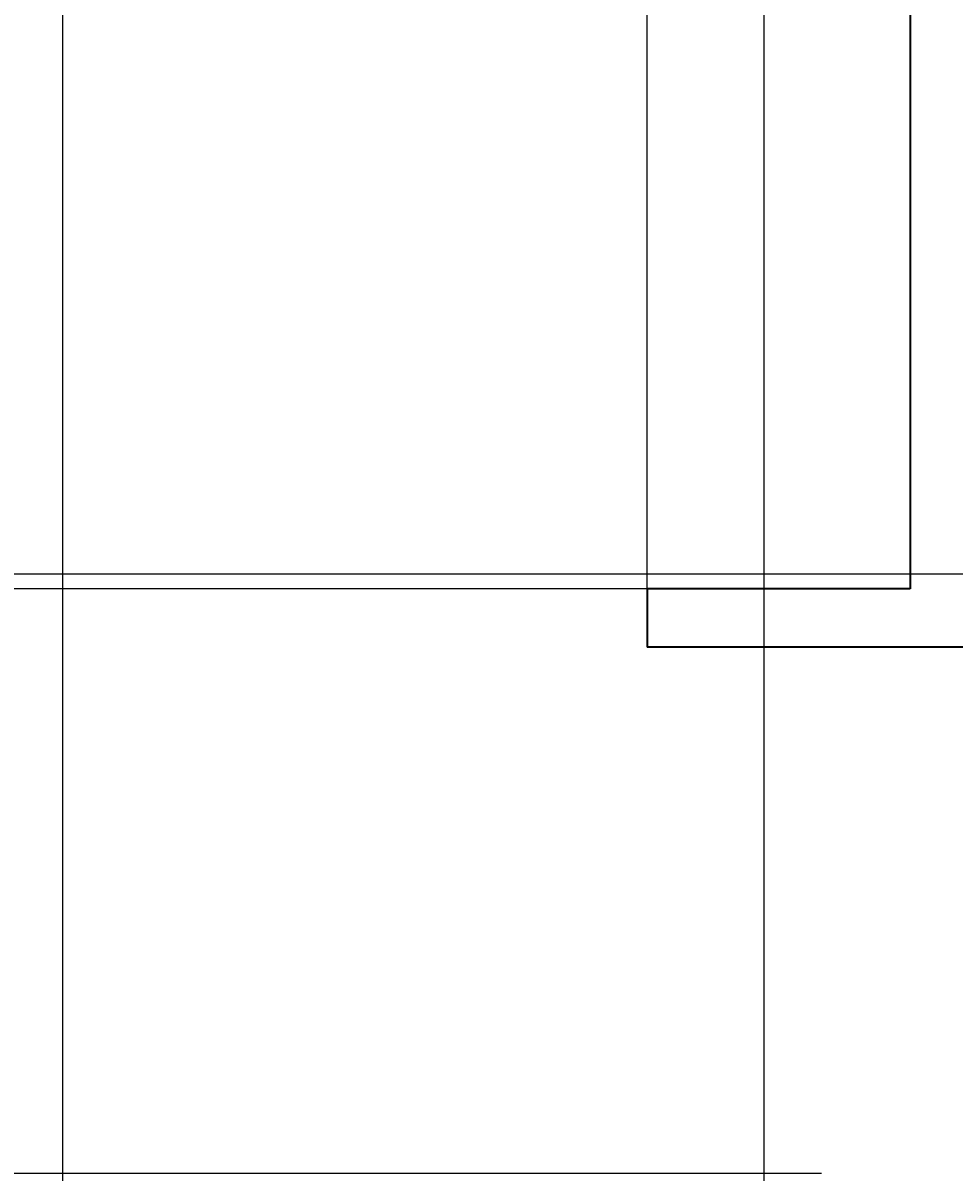
# Model space of a CAD drawing. Units: feet. Extents: x 105 to 1094, y -88 to 588.
# Tile 27 of 59: x 372 to 436, y 354 to 433. Entities that reach past the tile are written whole.
import ezdxf

# ---------------------------------------------------------------- set-up
doc = ezdxf.new("R2010")
doc.units = ezdxf.units.FT
doc.header["$MEASUREMENT"] = 0
doc.layers.add('A-ANNO-DIMS', color=2, linetype='Continuous', lineweight=18)
doc.layers.add('A-WALL', color=7, linetype='Continuous', lineweight=35)
doc.styles.get("Standard").update_dxf_attribs({"font": 'arial.ttf'})
doc.dimstyles.get("Standard").update_dxf_attribs({"dimtxt": 0.18, "dimasz": 0.18, "dimexe": 0.18, "dimexo": 0.0625, "dimgap": 0.09, "dimtad": 0, "dimtih": 1, "dimtoh": 1, "dimdec": 4, "dimzin": 0, "dimdsep": 46, "dimtxsty": 'Standard', "dimcen": 0.09, "dimadec": 0, "dimazin": 0, "dimtfac": 1, "dimtdec": 4, "dimtofl": 0, "dimtmove": 0, "dimatfit": 3, "dimfxl": 1, "dimtolj": 1, "dimtzin": 0, "dimarcsym": 0})

# ---------------------------------------------------------------- blocks, each defined once
blk = doc.blocks.new('*D21')
at = {"layer": 'A-ANNO-DIMS', "color": 0, "lineweight": -2, "transparency": 16777216}
for p, q in [((849.626, 543.081), (105.458, 543.081)), ((105.638, 542.901), (105.638, 250.263)), ((105.638, -42.739), (105.638, 249.899)), ((849.626, -42.919), (105.458, -42.919))]:
    blk.add_line(p, q, dxfattribs=at)
at = {"layer": 'A-ANNO-DIMS', "color": 0, "transparency": 16777216}
for points in [[(105.608, 542.901), (105.668, 542.901), (105.638, 543.081)], [(105.608, -42.739), (105.668, -42.739), (105.638, -42.919)]]:
    blk.add_solid(points, dxfattribs=at)
at = {"layer": 'Defpoints', "color": 0, "transparency": 16777216}
for p in [(105.638, 543.081), (849.688, 543.081), (849.688, -42.919)]:
    blk.add_point(p, dxfattribs=at)
at = {"layer": 'A-ANNO-DIMS', "color": 0, "transparency": 16777216, "insert": (105.638, 250.081), "char_height": 0.18, "attachment_point": 5}
blk.add_mtext('\\A1;586', dxfattribs=at)
blk = doc.blocks.new('*D33')
at = {"layer": 'A-ANNO-DIMS', "color": 0, "lineweight": -2, "transparency": 16777216}
for p, q in [((646.626, 395.081), (105.458, 395.081)), ((105.638, 394.901), (105.638, 345.263)), ((105.638, 295.261), (105.638, 344.899)), ((646.626, 295.081), (105.458, 295.081))]:
    blk.add_line(p, q, dxfattribs=at)
at = {"layer": 'A-ANNO-DIMS', "color": 0, "transparency": 16777216}
for points in [[(105.608, 394.901), (105.668, 394.901), (105.638, 395.081)], [(105.608, 295.261), (105.668, 295.261), (105.638, 295.081)]]:
    blk.add_solid(points, dxfattribs=at)
at = {"layer": 'Defpoints', "color": 0, "transparency": 16777216}
for p in [(646.688, 395.081), (105.638, 295.081), (646.688, 295.081)]:
    blk.add_point(p, dxfattribs=at)
at = {"layer": 'A-ANNO-DIMS', "color": 0, "transparency": 16777216, "insert": (105.638, 345.081), "char_height": 0.18, "attachment_point": 5}
blk.add_mtext('\\A1;100', dxfattribs=at)
blk = doc.blocks.new('*D51')
at = {"layer": 'A-ANNO-DIMS', "color": 0, "lineweight": -2, "transparency": 16777216}
for p, q in [((432.626, 394.081), (105.458, 394.081)), ((105.638, 393.901), (105.638, 374.263)), ((105.638, 354.261), (105.638, 373.899)), ((426.626, 354.081), (105.458, 354.081))]:
    blk.add_line(p, q, dxfattribs=at)
at = {"layer": 'A-ANNO-DIMS', "color": 0, "transparency": 16777216}
for points in [[(105.608, 393.901), (105.668, 393.901), (105.638, 394.081)], [(105.608, 354.261), (105.668, 354.261), (105.638, 354.081)]]:
    blk.add_solid(points, dxfattribs=at)
at = {"layer": 'Defpoints', "color": 0, "transparency": 16777216}
for p in [(432.688, 394.081), (105.638, 354.081), (426.688, 354.081)]:
    blk.add_point(p, dxfattribs=at)
at = {"layer": 'A-ANNO-DIMS', "color": 0, "transparency": 16777216, "insert": (105.638, 374.081), "char_height": 0.18, "attachment_point": 5}
blk.add_mtext('\\A1;40', dxfattribs=at)
blk = doc.blocks.new('*D52')
at = {"layer": 'A-ANNO-DIMS', "color": 0, "lineweight": -2, "transparency": 16777216}
for p, q in [((414.688, 394.144), (414.688, 588.311)), ((414.868, 588.131), (423.478, 588.131)), ((432.508, 588.131), (423.899, 588.131)), ((432.688, 394.144), (432.688, 588.311))]:
    blk.add_line(p, q, dxfattribs=at)
at = {"layer": 'A-ANNO-DIMS', "color": 0, "transparency": 16777216}
for points in [[(414.868, 588.161), (414.868, 588.101), (414.688, 588.131)], [(432.508, 588.161), (432.508, 588.101), (432.688, 588.131)]]:
    blk.add_solid(points, dxfattribs=at)
at = {"layer": 'Defpoints', "color": 0, "transparency": 16777216}
for p in [(414.688, 588.131), (414.688, 394.081), (432.688, 394.081)]:
    blk.add_point(p, dxfattribs=at)
at = {"layer": 'A-ANNO-DIMS', "color": 0, "transparency": 16777216, "insert": (423.688, 588.131), "char_height": 0.18, "attachment_point": 5}
blk.add_mtext('\\A1;18', dxfattribs=at)
blk = doc.blocks.new('*D53')
at = {"layer": 'A-ANNO-DIMS', "color": 0, "lineweight": -2, "transparency": 16777216}
for p, q in [((365.688, 394.144), (365.688, 588.311)), ((365.868, 588.131), (389.966, 588.131)), ((414.508, 588.131), (390.411, 588.131)), ((414.688, 394.144), (414.688, 588.311))]:
    blk.add_line(p, q, dxfattribs=at)
at = {"layer": 'A-ANNO-DIMS', "color": 0, "transparency": 16777216}
for points in [[(365.868, 588.161), (365.868, 588.101), (365.688, 588.131)], [(414.508, 588.161), (414.508, 588.101), (414.688, 588.131)]]:
    blk.add_solid(points, dxfattribs=at)
at = {"layer": 'Defpoints', "color": 0, "transparency": 16777216}
for p in [(365.688, 588.131), (365.688, 394.081), (414.688, 394.081)]:
    blk.add_point(p, dxfattribs=at)
at = {"layer": 'A-ANNO-DIMS', "color": 0, "transparency": 16777216, "insert": (390.188, 588.131), "char_height": 0.18, "attachment_point": 5}
blk.add_mtext('\\A1;49', dxfattribs=at)
blk = doc.blocks.new('*D56')
at = {"layer": 'A-ANNO-DIMS', "color": 0, "lineweight": -2, "transparency": 16777216}
for p, q in [((374.688, 252.144), (374.688, 588.311)), ((374.868, 588.131), (398.466, 588.131)), ((422.508, 588.131), (398.911, 588.131)), ((422.688, 252.144), (422.688, 588.311))]:
    blk.add_line(p, q, dxfattribs=at)
at = {"layer": 'A-ANNO-DIMS', "color": 0, "transparency": 16777216}
for points in [[(374.868, 588.161), (374.868, 588.101), (374.688, 588.131)], [(422.508, 588.161), (422.508, 588.101), (422.688, 588.131)]]:
    blk.add_solid(points, dxfattribs=at)
at = {"layer": 'Defpoints', "color": 0, "transparency": 16777216}
for p in [(422.688, 588.131), (374.688, 252.081), (422.688, 252.081)]:
    blk.add_point(p, dxfattribs=at)
at = {"layer": 'A-ANNO-DIMS', "color": 0, "transparency": 16777216, "insert": (398.688, 588.131), "char_height": 0.18, "attachment_point": 5}
blk.add_mtext('\\A1;48', dxfattribs=at)

msp = doc.modelspace()

# ---------------------------------------------------------------- linework, layer by layer
at = {"layer": 'A-WALL'}
for p, q in [((432.6883, 491.0812), (432.6883, 394.0812)), ((432.6883, 394.0812), (414.6883, 394.0812)), ((414.6883, 394.0812), (414.6883, 390.0812)), ((436.6883, 390.0812), (414.6883, 390.0812))]:
    msp.add_line(p, q, dxfattribs=at)

# ---------------------------------------------------------------- dimensions: what is measured, and where the dimension line sits
at = {"layer": 'A-ANNO-DIMS'}
for base, p1, p2, picture, middle in [((365.6883, 588.1312), (414.6883, 394.0812), (365.6883, 394.0812), '*D53', (390.1883, 588.1312)), ((422.6883, 588.1312), (374.6883, 252.0812), (422.6883, 252.0812), '*D56', (398.6883, 588.1312)), ((414.6883, 588.1312), (432.6883, 394.0812), (414.6883, 394.0812), '*D52', (423.6883, 588.1312))]:
    dim = msp.add_linear_dim(base=base, p1=p1, p2=p2, dimstyle='Standard', override={"dimdec": 0, "dimlfac": 1, "dimrnd": 0, "dimzin": 0, "dimdsep": 46, "dimlunit": 2}, dxfattribs=at)
    dim.commit()
    dim.dimension.update_dxf_attribs({"geometry": picture, "text_midpoint": middle})
for base, p1, p2, picture, middle in [((105.6383, 543.0812), (849.6883, -42.9188), (849.6883, 543.0812), '*D21', (105.6383, 250.0812)), ((105.6383, 295.0812), (646.6883, 395.0812), (646.6883, 295.0812), '*D33', (105.6383, 345.0812)), ((105.6383, 354.0812), (432.6883, 394.0812), (426.6883, 354.0812), '*D51', (105.6383, 374.0812))]:
    dim = msp.add_linear_dim(base=base, p1=p1, p2=p2, angle=90, dimstyle='Standard', override={"dimdec": 0, "dimlfac": 1, "dimrnd": 0, "dimzin": 0, "dimdsep": 46, "dimlunit": 2}, dxfattribs=at)
    dim.commit()
    dim.dimension.update_dxf_attribs({"geometry": picture, "text_midpoint": middle})

doc.saveas('drawing.dxf')
